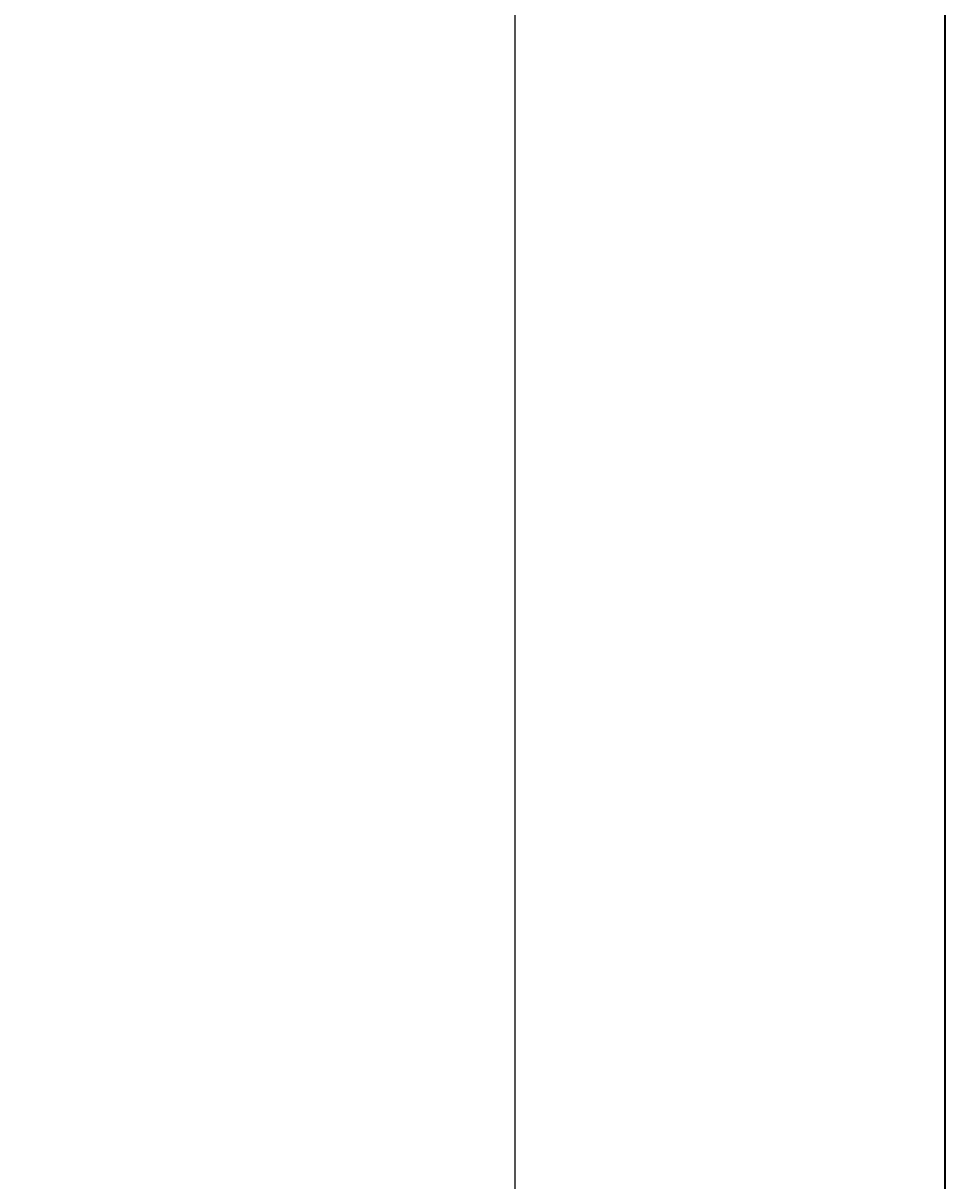
# Model space of a CAD drawing. Units: inches. Extents: x 1962 to 2771, y 1245 to 2660.
# Tile 21 of 114: x 2661 to 2771, y 1692 to 1831. Entities that reach past the tile are written whole.
import ezdxf

# ---------------------------------------------------------------- set-up
doc = ezdxf.new("R2010")
doc.units = ezdxf.units.IN
doc.layers.add('A-ANNO-DIMS', color=2, linetype='Continuous', lineweight=18)
doc.layers.add('A-ANNO-TTLB', color=7, linetype='Continuous', lineweight=35)
doc.styles.get("Standard").update_dxf_attribs({"font": 'arial.ttf'})
doc.dimstyles.get("Standard").update_dxf_attribs({"dimtxt": 0.18, "dimasz": 0.18, "dimexe": 0.18, "dimexo": 0.0625, "dimgap": 0.09, "dimtad": 0, "dimtih": 1, "dimtoh": 1, "dimdec": 4, "dimzin": 0, "dimdsep": 46, "dimtxsty": 'Standard', "dimcen": 0.09, "dimadec": 0, "dimazin": 0, "dimtfac": 1, "dimtdec": 4, "dimtofl": 0, "dimtmove": 0, "dimatfit": 3, "dimfxl": 1, "dimtolj": 1, "dimtzin": 0, "dimarcsym": 0})

# ---------------------------------------------------------------- blocks, each defined once
blk = doc.blocks.new('*D42')
at = {"layer": 'A-ANNO-DIMS', "color": 0, "lineweight": -2, "transparency": 16777216}
for p, q in [((2660.87, 2524.34), (2719.94, 2524.34)), ((2719.76, 2524.16), (2719.76, 1979.28)), ((2719.76, 1434.02), (2719.76, 1978.91)), ((2660.87, 1433.84), (2719.94, 1433.84))]:
    blk.add_line(p, q, dxfattribs=at)
at = {"layer": 'A-ANNO-DIMS', "color": 0, "transparency": 16777216}
for points in [[(2719.73, 2524.16), (2719.79, 2524.16), (2719.76, 2524.34)], [(2719.73, 1434.02), (2719.79, 1434.02), (2719.76, 1433.84)]]:
    blk.add_solid(points, dxfattribs=at)
at = {"layer": 'Defpoints', "color": 0, "transparency": 16777216}
for p in [(2660.81, 2524.34), (2719.76, 2524.34), (2660.81, 1433.84)]:
    blk.add_point(p, dxfattribs=at)
at = {"layer": 'A-ANNO-DIMS', "color": 0, "transparency": 16777216, "insert": (2719.76, 1979.09), "char_height": 0.18, "attachment_point": 5}
blk.add_mtext('\\A1;1090.5', dxfattribs=at)

msp = doc.modelspace()

# ---------------------------------------------------------------- linework, layer by layer
at = {"layer": 'A-ANNO-TTLB'}
msp.add_lwpolyline([(1961.7365, 2660.2579), (2771.213, 2660.2579), (2771.213, 1244.5817), (1961.7365, 1244.5817)], close=True, dxfattribs=at)

# ---------------------------------------------------------------- dimensions: what is measured, and where the dimension line sits
at = {"layer": 'A-ANNO-DIMS'}
dim = msp.add_linear_dim(base=(2719.7574, 2524.3437), p1=(2660.8074, 1433.8437), p2=(2660.8074, 2524.3437), angle=90, dimstyle='Standard', override={"dimdec": 1, "dimlfac": 1, "dimrnd": 0, "dimzin": 0, "dimdsep": 46, "dimlunit": 2}, dxfattribs=at)
dim.commit()
dim.dimension.update_dxf_attribs({"geometry": '*D42', "text_midpoint": (2719.7574, 1979.0937)})

doc.saveas('drawing.dxf')
